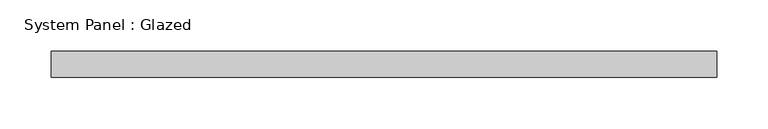
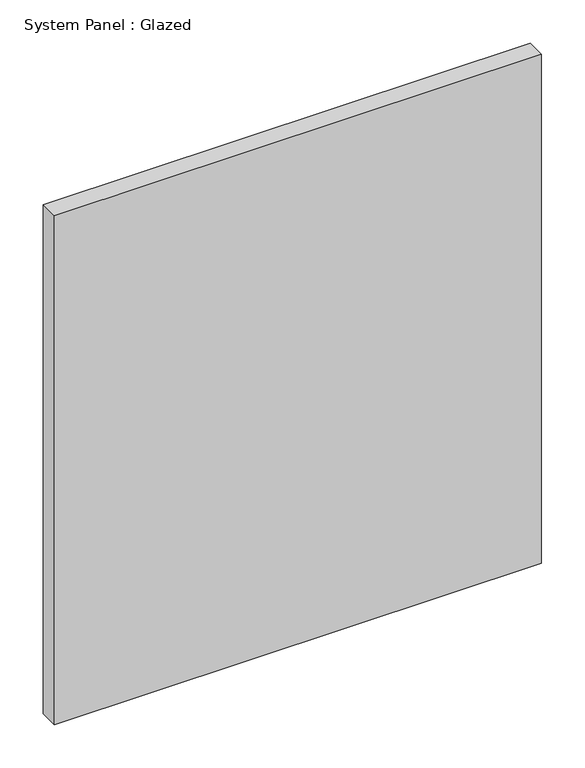
"""IFC4 building model written with IfcOpenShell, lengths in millimetres: plate geometry, System Panel : Glazed."""

from ifc_helpers import new_model, si_unit, origin, origin_with_axes, place, context, project, spatial, polyline, outline, extrude, source, transform, mapped, element, save


def system_panel_glazed_c2563f89(model_context):
    return source(origin(), model_context, "Body", "SweptSolid", [
        extrude(outline(polyline([(323.85, 19.05), (-323.85, 19.05), (-323.85, 44.45), (323.85, 44.45), (323.85, 19.05)])), origin_with_axes(), (0.0, 0.0, 1.0), 716.2173296),
    ])


if __name__ == "__main__":
    model = new_model("IFC4")
    model_context = context("Model", 3, world=origin())
    ifc_project = project(units=[si_unit("LENGTHUNIT", "METRE", prefix="MILLI")], contexts=[model_context])
    site = spatial("IfcSite", under=ifc_project)
    building = spatial("IfcBuilding", under=site)
    placement = place(None, origin())
    system_panel_glazed_shape = system_panel_glazed_c2563f89(model_context)
    element("IfcPlate", 1, ObjectType="System Panel : Glazed", at=placement, inside=building, context=model_context, shape_type="MappedRepresentation", body=[
        mapped(system_panel_glazed_shape, transform((0.0, 0.0, 0.0), x_axis=(1.0, 0.0, 0.0), y_axis=(0.0, 1.0, 0.0), z_axis=(0.0, 0.0, 1.0))),
    ])
    save(model, "model.ifc")

# Revit data of these elements
# Type "System Panel : Glazed"
#   Construction Type Id = "GSP4R"
#   Analytic Construction = "1/8 in Pilkington single glazing"
#   Visual Light Transmittance = 0.9
#   Solar Heat Gain Coefficient = 0.86
#   Heat Transfer Coefficient (U) = 1.18115 BTU/(h·ft²·°F)
#   Define Thermal Properties by = 1
# Element 1 (IfcPlate, "System Panel : Glazed")
#   Materials on its faces: "Glass"
# Materials
#   "Glass": class "Glass", colour RGB 0 128 192, transparency 0.75, Description = "Soda Lime Glass", Cost = 0
